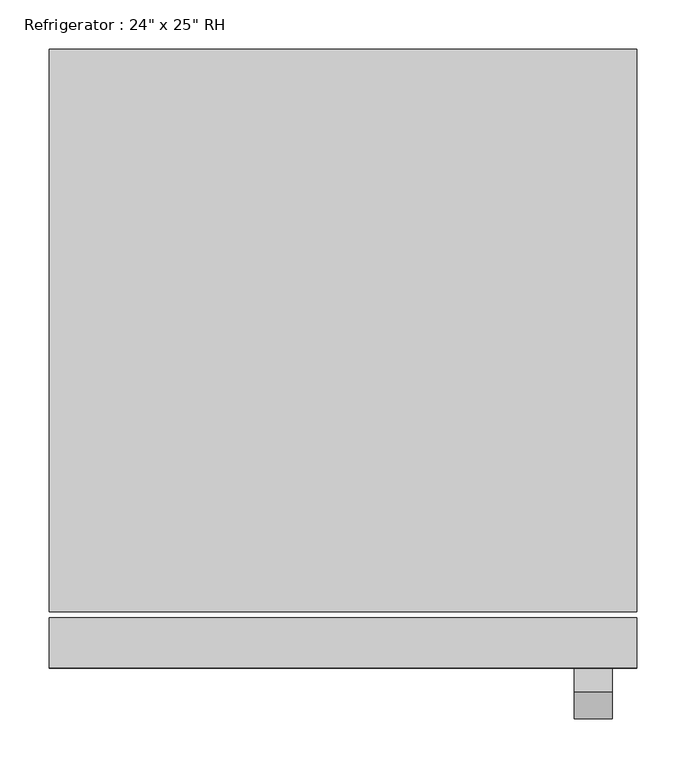
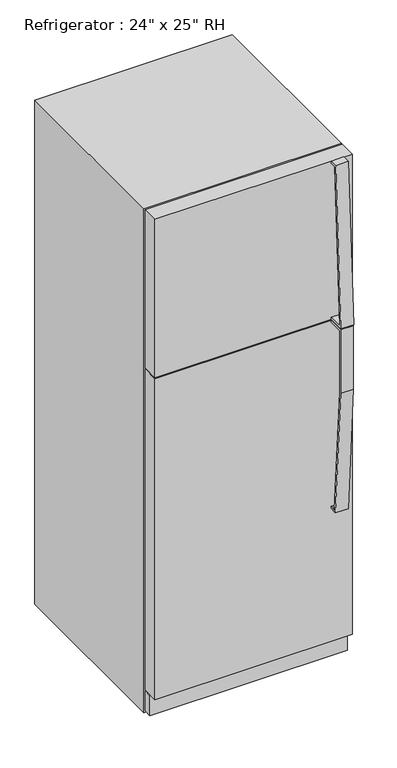
"""IFC4 building model written with IfcOpenShell, lengths in millimetres: proxy geometry."""

from ifc_helpers import new_model, si_unit, frame, origin, origin_with_axes, place, context, project, spatial, polyline, outline, extrude, source, transform, mapped, element, save


def proxy_66164f77(model_context):
    return source(origin(), model_context, "Body", "SweptSolid", [
        extrude(outline(polyline([(-329.0010285, 1096.9625), (-373.4510285, 1096.9625), (-373.4510285, 900.3342469), (-345.9723987, 507.3715334), (-329.0010285, 507.3715334), (-329.0010285, 501.0370017), (-351.8949512, 501.0370017), (-379.8010285, 900.1125), (-379.8010285, 1103.3125), (-329.0010285, 1103.3125), (-329.0010285, 1096.9625)])), frame((234.95, 0.0, 0.0), z_axis=(1.0, 0.0, 0.0), x_axis=(0.0, 1.0, 0.0)), (0.0, 0.0, 1.0), 38.4332978),
        extrude(outline(polyline([(-353.839413, 1612.9), (-329.7780855, 1612.9), (-329.7780855, 1606.55), (-348.6263449, 1606.55), (-374.5007207, 1112.8375), (-329.7780855, 1112.8375), (-329.7780855, 1106.4875), (-380.3793675, 1106.4875), (-353.839413, 1612.9)])), frame((234.95, 0.0, 0.0), z_axis=(1.0, 0.0, 0.0), x_axis=(0.0, 1.0, 0.0)), (0.0, 0.0, 1.0), 38.4332978),
        extrude(outline(polyline([(298.45, -278.2010285), (298.45, -303.6010285), (-298.45, -303.6010285), (-298.45, -278.2010285), (298.45, -278.2010285)])), frame((0.0, 0.0, 9.3816357), z_axis=(0.0, 0.0, 1.0), x_axis=(1.0, 0.0, 0.0)), (0.0, 0.0, 1.0), 63.5),
        extrude(outline(polyline([(298.45, -278.2010285), (298.45, -329.0010285), (-298.45, -329.0010285), (-298.45, -278.2010285), (298.45, -278.2010285)])), frame((0.0, 0.0, 76.2), z_axis=(0.0, 0.0, 1.0), x_axis=(1.0, 0.0, 0.0)), (0.0, 0.0, 1.0), 1027.1125),
        extrude(outline(polyline([(298.45, -278.2010285), (298.45, -329.0010285), (-298.45, -329.0010285), (-298.45, -278.2010285), (298.45, -278.2010285)])), frame((0.0, 0.0, 1106.4875), z_axis=(0.0, 0.0, 1.0), x_axis=(1.0, 0.0, 0.0)), (0.0, 0.0, 1.0), 506.4125),
        extrude(outline(polyline([(298.45, 299.6489715), (298.45, -271.8510285), (-298.45, -271.8510285), (-298.45, 299.6489715), (298.45, 299.6489715)])), origin_with_axes(), (0.0, 0.0, 1.0), 1612.9),
    ])


if __name__ == "__main__":
    model = new_model("IFC4")
    model_context = context("Model", 3, world=origin())
    ifc_project = project(units=[si_unit("LENGTHUNIT", "METRE", prefix="MILLI")], contexts=[model_context])
    site = spatial("IfcSite", under=ifc_project)
    building = spatial("IfcBuilding", under=site)
    placement = place(None, origin())
    proxy_shape = proxy_66164f77(model_context)
    element("IfcBuildingElementProxy", 1, Name="Refrigerator : 24\" x 25\" RH", ObjectType="Refrigerator : 24\" x 25\" RH", at=placement, inside=building, context=model_context, shape_type="MappedRepresentation", body=[
        mapped(proxy_shape, transform((0.0, 0.0, 0.0), x_axis=(1.0, 0.0, 0.0), y_axis=(0.0, 1.0, 0.0), z_axis=(0.0, 0.0, 1.0))),
    ])
    save(model, "model.ifc")

# Revit data of these elements
# Type "Refrigerator : 24\" x 25\" RH"
#   Label = "REF."
#   Assembly Code = "E1090400"
#   Depth = 2' - 0 3/4"
#   Handle = 1' - 9"
#   Height = 5' - 3 1/2"
#   Rear Clearance = 0' - 2"
#   Top Door Height = 1' - 8"
#   Width = 1' - 11 1/2"
#   Material = Steel, Paint Finish, Ivory, Glossy
#   Default Elevation = 0
# Element 1 (IfcBuildingElementProxy, "Refrigerator : 24\" x 25\" RH")
#   Materials on its faces: "Steel, Paint Finish, Ivory, Glossy", "Steel, Chrome Plated"
# Materials
#   "Steel, Paint Finish, Ivory, Glossy": class "Metal", colour RGB 247 247 239, transparency 0, Description = "Steel, paint finish, ivory, glossy", Cost = 0
#   "Steel, Chrome Plated": class "Metal", colour RGB 17 17 17, transparency 0, Description = "Chromiuim plated steel", Cost = 0
